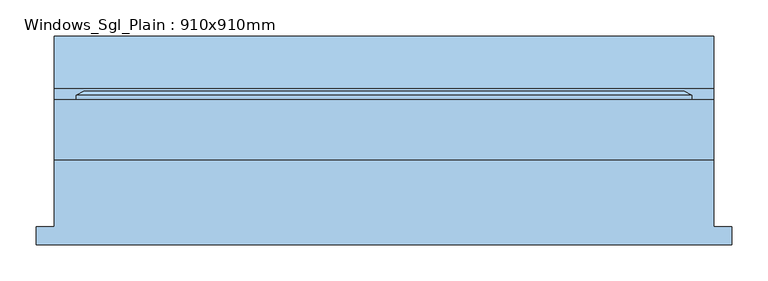
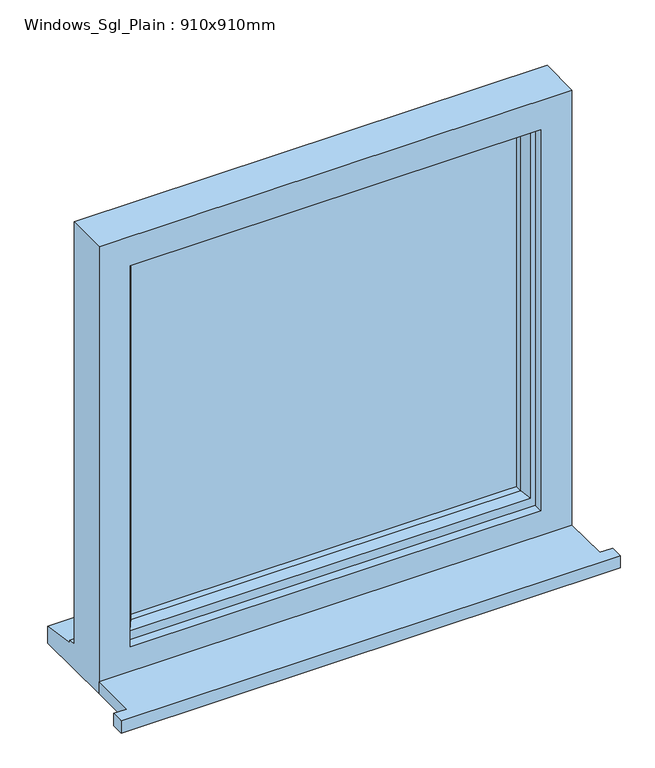
"""IFC4 building model written with IfcOpenShell, lengths in millimetres: window geometry, Windows_Sgl_Plain : 910x910mm."""

from ifc_helpers import new_model, si_unit, frame, origin, place, context, project, spatial, polyline, outline, extrude, faceted_brep, source, transform, mapped, element, save


def windows_sgl_plain_910x910mm_7835b02d(model_context):
    return source(origin(), model_context, "Body", "SolidModel", [
        extrude(outline(polyline([(-480.0, -129.0434322), (-480.0, -104.0434322), (-455.0, -104.0434322), (-455.0, -12.0434322), (455.0, -12.0434322), (455.0, -104.0434322), (480.0, -104.0434322), (480.0, -129.0434322), (-480.0, -129.0434322)])), frame((0.0, 0.0, 1200.0), z_axis=(0.0, 0.0, 1.0), x_axis=(1.0, 0.0, 0.0)), (0.0, 0.0, 1.0), 25.0),
        faceted_brep([(-455.0, -12.0434322, 1200.0), (455.0, -12.0434322, 1200.0), (455.0, -12.0434322, 2110.0), (-455.0, -12.0434322, 2110.0), (-395.0, -12.0434322, 2050.0), (395.0, -12.0434322, 2050.0), (395.0, -12.0434322, 1275.0), (-395.0, -12.0434322, 1275.0), (-455.0, 70.9565678, 2110.0), (-455.0, 70.9565678, 1251.0), (-455.0, 85.9565678, 1249.68767), (-455.0, 85.9565678, 1244.7449676), (-455.0, 158.4565678, 1233.8088847), (-455.0, 158.4565678, 1200.0), (455.0, 70.9565678, 2110.0), (455.0, 70.9565678, 1251.0), (-415.0, 70.9565678, 2070.0), (-415.0, 70.9565678, 1263.0), (415.0, 70.9565678, 1263.0), (415.0, 70.9565678, 2070.0), (-415.0, 5.9565678, 2070.0), (-415.0, 5.9565678, 1263.0), (415.0, 5.9565678, 2070.0), (415.0, 5.9565678, 1263.0), (-395.0, 5.9565678, 2050.0), (-395.0, 5.9565678, 1275.0), (395.0, 5.9565678, 1275.0), (395.0, 5.9565678, 2050.0), (455.0, 158.4565678, 1200.0), (455.0, 158.4565678, 1233.8088847), (455.0, 85.9565678, 1244.7449676), (455.0, 85.9565678, 1249.68767)], [[[0, 1, 2, 3], [4, 5, 6, 7]], [[0, 3, 8, 9, 10, 11, 12, 13]], [[9, 8, 14, 15], [16, 17, 18, 19]], [[17, 16, 20, 21]], [[20, 22, 23, 21], [24, 25, 26, 27]], [[24, 4, 7, 25]], [[3, 2, 14, 8]], [[16, 19, 22, 20]], [[5, 4, 24, 27]], [[15, 14, 2, 1, 28, 29, 30, 31]], [[19, 18, 23, 22]], [[5, 27, 26, 6]], [[28, 1, 0, 13]], [[29, 28, 13, 12]], [[30, 29, 12, 11]], [[31, 30, 11, 10]], [[15, 31, 10, 9]], [[21, 23, 18, 17]], [[7, 6, 26, 25]]]),
        extrude(outline(polyline([(385.0, 34.9565678), (-385.0, 34.9565678), (-385.0, 58.9565678), (385.0, 58.9565678), (385.0, 34.9565678)])), frame((0.0, 0.0, 1293.0), z_axis=(0.0, 0.0, 1.0), x_axis=(1.0, 0.0, 0.0)), (0.0, 0.0, 1.0), 747.0),
        faceted_brep([(-425.0, 70.9565678, 2080.0), (-425.0, 76.7300705, 2080.0), (-425.0, 76.7300705, 1253.0), (-425.0, 70.9565678, 1253.0), (-415.0, 5.9565678, 2070.0), (-415.0, 70.9565678, 2070.0), (-415.0, 70.9565678, 1263.0), (-415.0, 5.9565678, 1263.0), (-375.0, 20.4494677, 2030.0), (-385.1480377, 5.9565678, 2040.1480377), (-385.1480377, 5.9565678, 1292.8519623), (-375.0, 20.4494677, 1303.0), (-375.0, 34.9565678, 2030.0), (-375.0, 34.9565678, 1303.0), (-385.0, 58.9565678, 2040.0), (-385.0, 34.9565678, 2040.0), (-385.0, 34.9565678, 1293.0), (-385.0, 58.9565678, 1293.0), (-375.0, 76.7300705, 2030.0), (-375.0, 58.9565678, 2030.0), (-375.0, 58.9565678, 1303.0), (-375.0, 76.7300705, 1303.0), (-392.4457548, 82.5035732, 2047.4457548), (-392.4457548, 82.5035732, 1285.5542452), (-414.2153903, 82.5035732, 2069.2153903), (-414.2153903, 82.5035732, 1263.7846097), (425.0, 76.7300705, 1253.0), (425.0, 70.9565678, 1253.0), (415.0, 70.9565678, 1263.0), (415.0, 5.9565678, 1263.0), (385.1480377, 5.9565678, 1292.8519623), (375.0, 20.4494677, 1303.0), (375.0, 34.9565678, 1303.0), (385.0, 34.9565678, 1293.0), (385.0, 58.9565678, 1293.0), (375.0, 58.9565678, 1303.0), (375.0, 76.7300705, 1303.0), (392.4457548, 82.5035732, 1285.5542452), (414.2153903, 82.5035732, 1263.7846097), (425.0, 76.7300705, 2080.0), (425.0, 70.9565678, 2080.0), (415.0, 70.9565678, 2070.0), (415.0, 5.9565678, 2070.0), (385.1480377, 5.9565678, 2040.1480377), (375.0, 20.4494677, 2030.0), (375.0, 34.9565678, 2030.0), (385.0, 34.9565678, 2040.0), (385.0, 58.9565678, 2040.0), (375.0, 58.9565678, 2030.0), (375.0, 76.7300705, 2030.0), (392.4457548, 82.5035732, 2047.4457548), (414.2153903, 82.5035732, 2069.2153903)], [[[0, 1, 2, 3]], [[4, 5, 6, 7]], [[8, 9, 10, 11]], [[12, 8, 11, 13]], [[14, 15, 16, 17]], [[18, 19, 20, 21]], [[22, 18, 21, 23]], [[1, 24, 25, 2]], [[3, 2, 26, 27]], [[7, 6, 28, 29]], [[11, 10, 30, 31]], [[13, 11, 31, 32]], [[17, 16, 33, 34]], [[21, 20, 35, 36]], [[23, 21, 36, 37]], [[2, 25, 38, 26]], [[27, 26, 39, 40]], [[29, 28, 41, 42]], [[31, 30, 43, 44]], [[32, 31, 44, 45]], [[34, 33, 46, 47]], [[36, 35, 48, 49]], [[37, 36, 49, 50]], [[26, 38, 51, 39]], [[40, 39, 1, 0]], [[3, 27, 40, 0], [5, 41, 28, 6]], [[42, 41, 5, 4]], [[7, 29, 42, 4], [9, 43, 30, 10]], [[44, 43, 9, 8]], [[45, 44, 8, 12]], [[15, 46, 33, 16], [13, 32, 45, 12]], [[47, 46, 15, 14]], [[17, 34, 47, 14], [19, 48, 35, 20]], [[49, 48, 19, 18]], [[50, 49, 18, 22]], [[24, 51, 38, 25], [23, 37, 50, 22]], [[39, 51, 24, 1]]]),
    ])


if __name__ == "__main__":
    model = new_model("IFC4")
    model_context = context("Model", 3, world=origin())
    ifc_project = project(units=[si_unit("LENGTHUNIT", "METRE", prefix="MILLI")], contexts=[model_context])
    site = spatial("IfcSite", under=ifc_project)
    building = spatial("IfcBuilding", under=site)
    placement = place(None, origin())
    windows_sgl_plain_910x910mm_shape = windows_sgl_plain_910x910mm_7835b02d(model_context)
    element("IfcWindow", 1, ObjectType="Windows_Sgl_Plain : 910x910mm", at=placement, inside=building, context=model_context, shape_type="MappedRepresentation", body=[
        mapped(windows_sgl_plain_910x910mm_shape, transform((0.0, 0.0, 0.0), x_axis=(1.0, 0.0, 0.0), y_axis=(0.0, 1.0, 0.0), z_axis=(0.0, 0.0, 1.0))),
    ])
    save(model, "model.ifc")

# Revit data of these elements
# Type "Windows_Sgl_Plain : 910x910mm"
#   Type Mark = "44"
#   Operation = "SinglePanel"
#   Construction Type Id = "SGL"
#   Manufacturer = "Revit"
#   Keynote = "L10"
#   Analytic Construction = "Large single-glazed windows"
#   Wrap Layers (Ext) from Ext = 102.5 mm
#   Wrap Layers (Int) from Ext = 177.5 mm
#   Window Board Projection = 25 mm
#   Window Board Extension = 25 mm
#   Visual Light Transmittance = 0.9
#   Solar Heat Gain Coefficient = 0.86
#   Rough Width = 910 mm
#   Rough Height = 910 mm
#   Height = 910 mm
#   Width = 910 mm
#   Heat Transfer Coefficient (U) = 5.5617 W/(m²·K)
#   Glazing Thickness = 24 mm
#   FrameOffset - External = 50 mm
#   Frame Depth = 65 mm
#   Default Head Height = 2110 mm
#   Cill Depth = 87.5 mm
#   Cavity Closer Width = 50 mm
#   Cavity Closer Offset from Ext = 102.5 mm
#   Cavity Closer Depth = 85 mm
#   Define Thermal Properties by = 1
#   Vis - Cavity Closers = yes
#   Define Thermal Properties by = 1
#   Material Trim = Window Frame
#   Material Glass = Glass
#   Material Frame = Window Frame
#   Wall Closure = (empty or 0)
# Element 1 (IfcWindow, "Windows_Sgl_Plain : 910x910mm")
#   Materials on its faces: "Window Frame", "Glass"
# Materials
#   "Window Frame": colour RGB 249 249 249, transparency 0, Keynote = "L10", Cost = 0
#   "Glass": class "Glass", colour RGB 0 128 192, transparency 0.9, Description = "Soda Lime Glass", Cost = 0
